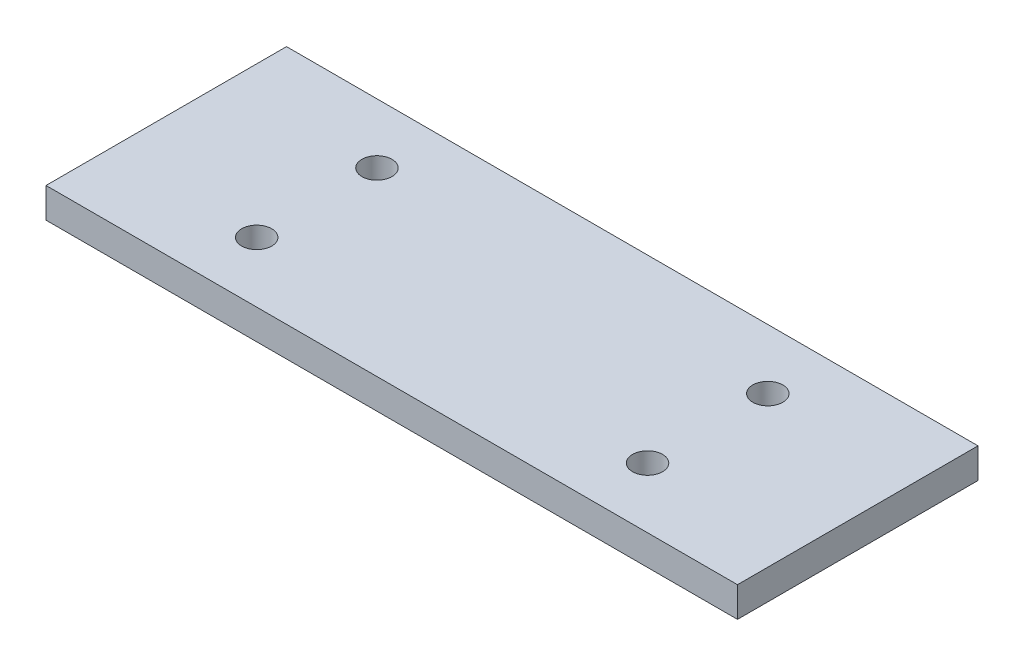
SolidWorks part; units mm, degrees
material "Plain Carbon Steel"
ref_plane "Front Plane" through (0, 0, 0) normal (0, 0, 1) x (1, 0, 0)
ref_plane "Top Plane" through (0, 0, 0) normal (0, 1, 0) x (1, 0, 0)
ref_plane "Right Plane" through (0, 0, 0) normal (1, 0, 0) x (0, 0, -1)
sketch "Base Plate Profile with 4 Holes" plane through (0, 0, 0) normal (0, 1, 0) x (1, 0, 0)
  line L0 (0, 0) -> (0, -43.6425) construction
  line L1 (-57.5, 20) -> (57.5, 20)
  line L2 (-57.5, 20) -> (-57.5, -20)
  line L3 (-57.5, -20) -> (57.5, -20)
  line L4 (57.5, 20) -> (57.5, -20)
  line L5 (-57.5, 20) -> (57.5, -20) construction
  line L6 (-57.5, -20) -> (57.5, 20) construction
  circle A0 centre (-32.5, 10.0414) radius 2.5
  circle A1 centre (-32.5, -9.9586) radius 2.5
  circle A2 centre (32.5, -9.9586) radius 2.5
  circle A3 centre (32.5, 10.0414) radius 2.5
  point P0 (0, 0)
  dimension "D2" = 5
  dimension "D1" = 40
  dimension "115" = 115
  dimension "D3" = 25
  dimension "D4" = 20
  dimension "D5" = 10.0414
extrude "Base Plate 115x40x5" add sketch "Base Plate Profile with 4 Holes" along normal blind 5
